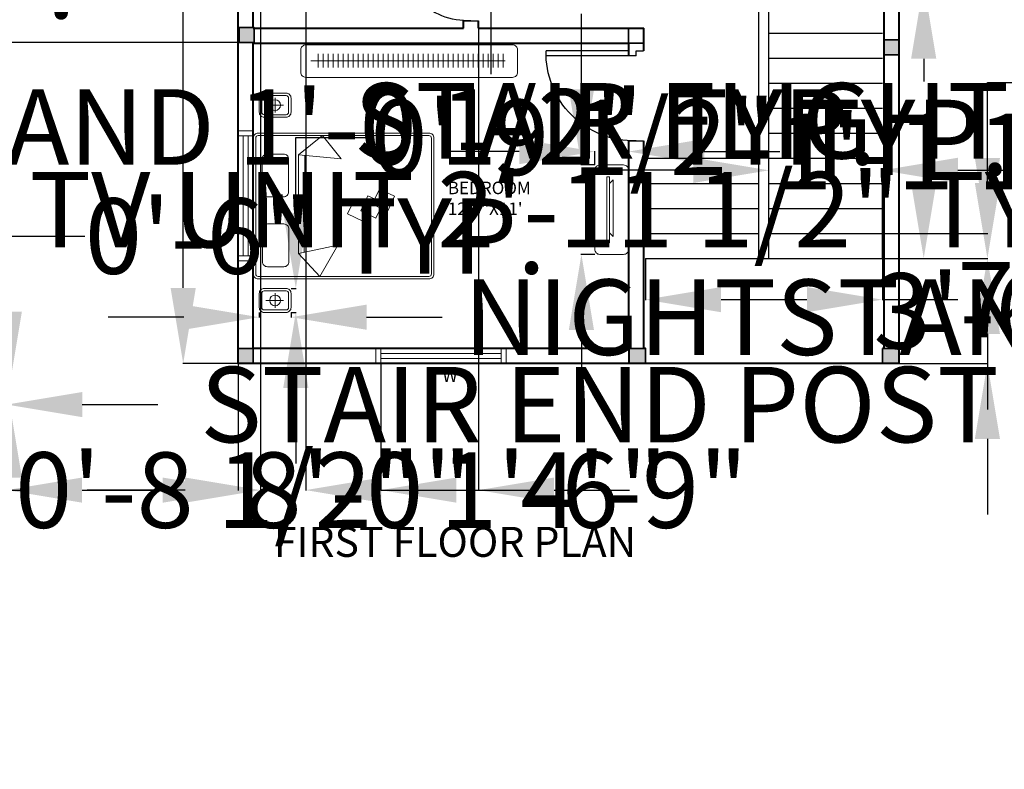
# Model space of a CAD drawing. Units: inches. Extents: x 7323 to 9737, y 2037 to 3322.
# Tile 7 of 19: x 8921 to 9314, y 2037 to 2337. Entities that reach past the tile are written whole.
import ezdxf

# ---------------------------------------------------------------- set-up
doc = ezdxf.new("R2010")
doc.units = ezdxf.units.IN
doc.header["$MEASUREMENT"] = 0
for name, color, linetype, lineweight in [('A-ANNO-DIMS', 2, 'Continuous', 18), ('A-ANNO-TEXT', 7, 'Continuous', 25), ('A-AREA-IDEN', 7, 'Continuous', 18), ('A-COLS', 1, 'Continuous', 35), ('A-DOOR', 4, 'Continuous', 25), ('A-FLOR-CASE', 9, 'Continuous', 20), ('A-FLOR-CASE-PATT', 8, 'Continuous', 13), ('A-FLOR-STRS', 7, 'Continuous', 25), ('A-FURN', 8, 'Continuous', 18), ('A-GLAZ', 4, 'Continuous', 18), ('A-WALL', 7, 'Continuous', 40)]:
    doc.layers.add(name, color=color, linetype=linetype, lineweight=lineweight)
doc.layers.add('A-COLS-PATT', color=18, linetype='Continuous', lineweight=13, true_color=0x000000)
doc.styles.get("Standard").update_dxf_attribs({"font": 'arial.ttf'})
doc.dimstyles.get("Standard").update_dxf_attribs({"dimtxt": 30.18, "dimasz": 30.18, "dimexe": 0.18, "dimexo": 0.0625, "dimgap": 0.09, "dimtad": 0, "dimtih": 1, "dimtoh": 1, "dimdec": 0, "dimzin": 0, "dimdsep": 46, "dimlunit": 3, "dimtxsty": 'Standard', "dimcen": 0.09, "dimadec": 0, "dimazin": 0, "dimtfac": 1, "dimtdec": 0, "dimtofl": 0, "dimtmove": 0, "dimatfit": 3, "dimfxl": 1, "dimtolj": 1, "dimtzin": 0, "dimarcsym": 0})

# ---------------------------------------------------------------- blocks, each defined once
blk = doc.blocks.new('*D11')
at = {"layer": 'A-ANNO-DIMS', "color": 0, "lineweight": -2, "transparency": 16777216}
for p, q in [((9007.88, 2687.3), (8985.8, 2687.3)), ((8985.98, 2657.12), (8985.98, 2458.79)), ((8985.98, 2229.48), (8985.98, 2427.8)), ((9007.88, 2199.3), (8985.8, 2199.3))]:
    blk.add_line(p, q, dxfattribs=at)
at = {"layer": 'A-ANNO-DIMS', "color": 0, "transparency": 16777216}
for points in [[(8980.95, 2657.12), (8991.01, 2657.12), (8985.98, 2687.3)], [(8980.95, 2229.48), (8991.01, 2229.48), (8985.98, 2199.3)]]:
    blk.add_solid(points, dxfattribs=at)
at = {"layer": 'Defpoints', "color": 0, "transparency": 16777216}
for p in [(9007.95, 2687.3), (8985.98, 2199.3), (9007.95, 2199.3)]:
    blk.add_point(p, dxfattribs=at)
at = {"layer": 'A-ANNO-DIMS', "color": 0, "transparency": 16777216, "insert": (8985.98, 2443.3), "char_height": 30.18, "attachment_point": 5}
blk.add_mtext('\\A1;40\'-8"', dxfattribs=at)
blk = doc.blocks.new('WIN-48')
for p, q in [((0, 0), (0, 6)), ((2, 0), (2, 6)), ((2, 4), (50, 4)), ((50, 0), (50, 6)), ((52, 0), (52, 6)), ((2, 2), (50, 2))]:
    blk.add_line(p, q)
blk = doc.blocks.new('STAIR-RETURN-FLIGHT')
for p, q in [((45.32, 110), (94.63, 110)), ((45.32, 0), (45.32, 110)), ((49.32, 0), (49.32, 110)), ((49.32, 100), (94.63, 100)), ((49.32, 90), (94.63, 90)), ((49.32, 80), (94.63, 80)), ((49.32, 70), (94.63, 70)), ((49.32, 60), (94.63, 60)), ((49.32, 50), (94.63, 50)), ((0, 40), (45.32, 40)), ((49.32, 40), (94.63, 40)), ((0, 30), (45.32, 30)), ((49.32, 30), (94.63, 30)), ((0, 20), (45.32, 20)), ((49.32, 20), (94.63, 20)), ((0, 10), (45.32, 10)), ((49.32, 10), (94.63, 10)), ((0, 0), (94.63, 0))]:
    blk.add_line(p, q)
blk = doc.blocks.new('DOOR-36')
for p, q in [((33.01, 39), (39.01, 39)), ((36.01, 5), (0.01, 5)), ((36.01, 5), (36.01, 3)), ((33.01, 3), (0.01, 3)), ((36.01, 3), (39.01, 3)), ((33.01, 0), (39.01, 0))]:
    blk.add_line(p, q)
blk.add_arc((35.01, 4), 35.01, 88.3634, 181.6366)
blk = doc.blocks.new('DOOR-30')
for p, q in [((27.01, 33), (33.01, 33)), ((30.01, 5), (0.01, 5)), ((30.01, 5), (30.01, 3)), ((27.01, 3), (0.01, 3)), ((30.01, 3), (33.01, 3)), ((27.01, 0), (33.01, 0))]:
    blk.add_line(p, q)
blk.add_arc((29.01, 4), 29.02, 88.0251, 181.9749)
blk = doc.blocks.new('MEDIA-CONSOLE')
for p, q in [((5.81, 28.29), (7.29, 29.79)), ((7.29, 29.79), (7.29, 7.16)), ((7.29, 7.16), (5.81, 8.58))]:
    blk.add_line(p, q)
blk.add_lwpolyline([(13.51, 33.75, 0.414214), (11.51, 35.75), (2, 35.75, 0.414214), (0, 33.75), (0, 2, 0.414214), (2, 0), (11.51, 0, 0.414214), (13.51, 2)], format="xyb", close=True)
blk.add_lwpolyline([(5.81, 30.96), (5.81, 30.96), (4.8, 30.96), (4.8, 30.96), (4.8, 4.61), (4.8, 4.61), (5.81, 4.61), (5.81, 4.61)], close=True)
blk = doc.blocks.new('NIGHTSTAND-COMPACT-II')
for p, q in [((2.65, 4.81), (9.72, 4.81)), ((6.35, 7.74), (6.35, 1.85))]:
    blk.add_line(p, q)
for points in [[(0, 7.61, -0.414214), (2, 9.61), (10.71, 9.61, -0.414214), (12.71, 7.61), (12.71, 2, -0.414214), (10.71, 0), (2, 0, -0.414214), (0, 2)], [(1, 7.61, -0.414214), (2, 8.61), (10.71, 8.61, -0.414214), (11.71, 7.61), (11.71, 2, -0.414214), (10.71, 1), (2, 1, -0.414214), (1, 2)]]:
    blk.add_lwpolyline(points, format="xyb", close=True)
blk.add_circle((6.35, 4.81), 2.16)
blk = doc.blocks.new('COL-PLAN-6IN')
blk.add_lwpolyline([(0, 6), (0, 6), (6.06, 6), (6.06, 6), (6.06, 0), (6.06, 0), (0, 0), (0, 0)], close=True)
blk = doc.blocks.new('COL-STAIR-END')
blk.add_lwpolyline([(0, 6), (6.74, 6), (6.74, 0), (0, 0)], close=True)
blk = doc.blocks.new('*D41')
at = {"layer": 'A-ANNO-DIMS', "color": 0, "lineweight": -2, "transparency": 16777216}
for p, q in [((8661.59, 2428.04), (8661.59, 2458.22)), ((8661.59, 2458.22), (8691.77, 2458.22)), ((8657.46, 2397.86), (8661.77, 2397.86)), ((8657.46, 2369.86), (8661.77, 2369.86)), ((8661.59, 2339.68), (8661.59, 2309.5))]:
    blk.add_line(p, q, dxfattribs=at)
at = {"layer": 'A-ANNO-DIMS', "color": 0, "transparency": 16777216}
for points in [[(8656.56, 2428.04), (8666.62, 2428.04), (8661.59, 2397.86)], [(8656.56, 2339.68), (8666.62, 2339.68), (8661.59, 2369.86)]]:
    blk.add_solid(points, dxfattribs=at)
at = {"layer": 'Defpoints', "color": 0, "transparency": 16777216}
for p in [(8657.39, 2397.86), (8661.59, 2397.86), (8657.39, 2369.86)]:
    blk.add_point(p, dxfattribs=at)
at = {"layer": 'A-ANNO-DIMS', "color": 0, "transparency": 16777216, "insert": (8945.06, 2458.22), "char_height": 30.18, "attachment_point": 5}
blk.add_mtext('\\A1;VENT WINDOW 2\'-4" TYP.', dxfattribs=at)
blk = doc.blocks.new('*D43')
at = {"layer": 'A-ANNO-DIMS', "color": 0, "lineweight": -2, "transparency": 16777216}
for p, q in [((9108.94, 2438.75), (9108.94, 2468.93)), ((9104.01, 2408.57), (9109.12, 2408.57)), ((9104.01, 2375.3), (9109.12, 2375.3)), ((9108.94, 2345.12), (9108.94, 2314.94))]:
    blk.add_line(p, q, dxfattribs=at)
at = {"layer": 'A-ANNO-DIMS', "color": 0, "transparency": 16777216}
for points in [[(9103.91, 2438.75), (9113.97, 2438.75), (9108.94, 2408.57)], [(9103.91, 2345.12), (9113.97, 2345.12), (9108.94, 2375.3)]]:
    blk.add_solid(points, dxfattribs=at)
at = {"layer": 'Defpoints', "color": 0, "transparency": 16777216}
for p in [(9103.95, 2408.57), (9108.94, 2408.57), (9103.95, 2375.3)]:
    blk.add_point(p, dxfattribs=at)
at = {"layer": 'A-ANNO-DIMS', "color": 0, "transparency": 16777216, "insert": (9108.94, 2391.93), "char_height": 30.18, "attachment_point": 5}
blk.add_mtext('\\A1;BATH DOOR 2\'-9 1/2" TYP.', dxfattribs=at)
blk = doc.blocks.new('*D44')
at = {"layer": 'A-ANNO-DIMS', "color": 0, "lineweight": -2, "transparency": 16777216}
for p, q in [((9070.67, 2375.23), (9070.67, 2370.12)), ((9103.95, 2375.23), (9103.95, 2370.12)), ((9040.49, 2370.3), (9010.31, 2370.3)), ((9134.13, 2370.3), (9164.31, 2370.3))]:
    blk.add_line(p, q, dxfattribs=at)
at = {"layer": 'A-ANNO-DIMS', "color": 0, "transparency": 16777216}
for points in [[(9040.49, 2375.33), (9040.49, 2365.27), (9070.67, 2370.3)], [(9134.13, 2375.33), (9134.13, 2365.27), (9103.95, 2370.3)]]:
    blk.add_solid(points, dxfattribs=at)
at = {"layer": 'Defpoints', "color": 0, "transparency": 16777216}
for p in [(9070.67, 2375.3), (9103.95, 2375.3), (9103.95, 2370.3)]:
    blk.add_point(p, dxfattribs=at)
at = {"layer": 'A-ANNO-DIMS', "color": 0, "transparency": 16777216, "insert": (9291.8, 2370.3), "char_height": 30.18, "attachment_point": 5}
blk.add_mtext('\\A1;2\'-9 1/2" TYP.', dxfattribs=at)
blk = doc.blocks.new('*D49')
at = {"layer": 'A-ANNO-DIMS', "color": 0, "lineweight": -2, "transparency": 16777216}
for p, q in [((8908.77, 2183.8), (8908.77, 2182.67)), ((8915.5, 2183.8), (8915.5, 2182.67)), ((8878.59, 2182.85), (8848.41, 2182.85)), ((8945.68, 2182.85), (8975.86, 2182.85))]:
    blk.add_line(p, q, dxfattribs=at)
at = {"layer": 'A-ANNO-DIMS', "color": 0, "transparency": 16777216}
for points in [[(8878.59, 2187.88), (8878.59, 2177.82), (8908.77, 2182.85)], [(8945.68, 2187.88), (8945.68, 2177.82), (8915.5, 2182.85)]]:
    blk.add_solid(points, dxfattribs=at)
at = {"layer": 'Defpoints', "color": 0, "transparency": 16777216}
for p in [(8908.77, 2183.86), (8915.5, 2183.86), (8915.5, 2182.85)]:
    blk.add_point(p, dxfattribs=at)
at = {"layer": 'A-ANNO-DIMS', "color": 0, "transparency": 16777216, "insert": (9284.58, 2182.85), "char_height": 30.18, "attachment_point": 5}
blk.add_mtext('\\A1;STAIR END POST 0\'-6 1/2" TYP.', dxfattribs=at)
blk = doc.blocks.new('*D50')
at = {"layer": 'A-ANNO-DIMS', "color": 0, "lineweight": -2, "transparency": 16777216}
for p, q in [((8916.51, 2220.04), (8916.51, 2250.22)), ((8916.51, 2250.22), (8946.69, 2250.22)), ((8915.57, 2189.86), (8916.69, 2189.86)), ((8915.57, 2183.86), (8916.69, 2183.86)), ((8916.51, 2153.68), (8916.51, 2123.5))]:
    blk.add_line(p, q, dxfattribs=at)
at = {"layer": 'A-ANNO-DIMS', "color": 0, "transparency": 16777216}
for points in [[(8911.48, 2220.04), (8921.54, 2220.04), (8916.51, 2189.86)], [(8911.48, 2153.68), (8921.54, 2153.68), (8916.51, 2183.86)]]:
    blk.add_solid(points, dxfattribs=at)
at = {"layer": 'Defpoints', "color": 0, "transparency": 16777216}
for p in [(8915.5, 2189.86), (8916.51, 2189.86), (8915.5, 2183.86)]:
    blk.add_point(p, dxfattribs=at)
at = {"layer": 'A-ANNO-DIMS', "color": 0, "transparency": 16777216, "insert": (9038.77, 2250.22), "char_height": 30.18, "attachment_point": 5}
blk.add_mtext('\\A1;0\'-6" TYP.', dxfattribs=at)
blk = doc.blocks.new('*D55')
at = {"layer": 'A-ANNO-DIMS', "color": 0, "lineweight": -2, "transparency": 16777216}
for p, q in [((9265.38, 2351.3), (9282, 2351.3)), ((9281.82, 2321.12), (9281.82, 2311.99)), ((9281.82, 2271.48), (9281.82, 2280.6)), ((9265.38, 2241.3), (9282, 2241.3))]:
    blk.add_line(p, q, dxfattribs=at)
at = {"layer": 'A-ANNO-DIMS', "color": 0, "transparency": 16777216}
for points in [[(9276.79, 2321.12), (9286.85, 2321.12), (9281.82, 2351.3)], [(9276.79, 2271.48), (9286.85, 2271.48), (9281.82, 2241.3)]]:
    blk.add_solid(points, dxfattribs=at)
at = {"layer": 'Defpoints', "color": 0, "transparency": 16777216}
for p in [(9265.32, 2351.3), (9281.82, 2351.3), (9265.32, 2241.3)]:
    blk.add_point(p, dxfattribs=at)
at = {"layer": 'A-ANNO-DIMS', "color": 0, "transparency": 16777216, "insert": (9281.82, 2296.3), "char_height": 30.18, "attachment_point": 5}
blk.add_mtext('\\A1;STAIR FLIGHT 9\'-2" TYP.', dxfattribs=at)
blk = doc.blocks.new('*D56')
at = {"layer": 'A-ANNO-DIMS', "color": 0, "lineweight": -2, "transparency": 16777216}
for p, q in [((9170.68, 2241.23), (9170.68, 2224.62)), ((9265.32, 2241.23), (9265.32, 2224.62)), ((9200.86, 2224.8), (9235.14, 2224.8)), ((9265.32, 2224.8), (9295.5, 2224.8))]:
    blk.add_line(p, q, dxfattribs=at)
at = {"layer": 'A-ANNO-DIMS', "color": 0, "transparency": 16777216}
for points in [[(9200.86, 2229.83), (9200.86, 2219.77), (9170.68, 2224.8)], [(9235.14, 2229.83), (9235.14, 2219.77), (9265.32, 2224.8)]]:
    blk.add_solid(points, dxfattribs=at)
at = {"layer": 'Defpoints', "color": 0, "transparency": 16777216}
for p in [(9170.68, 2241.3), (9265.32, 2241.3), (9265.32, 2224.8)]:
    blk.add_point(p, dxfattribs=at)
at = {"layer": 'A-ANNO-DIMS', "color": 0, "transparency": 16777216, "insert": (9434.33, 2224.8), "char_height": 30.18, "attachment_point": 5}
blk.add_mtext('\\A1;7\'-10 1/2" TYP.', dxfattribs=at)
blk = doc.blocks.new('*D67')
at = {"layer": 'A-ANNO-DIMS', "color": 0, "lineweight": -2, "transparency": 16777216}
for p, q in [((9145.07, 2308.82), (9145.07, 2339)), ((9150.37, 2278.64), (9144.89, 2278.64)), ((9150.37, 2242.89), (9144.89, 2242.89)), ((9145.07, 2212.71), (9145.07, 2182.53))]:
    blk.add_line(p, q, dxfattribs=at)
at = {"layer": 'A-ANNO-DIMS', "color": 0, "transparency": 16777216}
for points in [[(9140.04, 2308.82), (9150.1, 2308.82), (9145.07, 2278.64)], [(9140.04, 2212.71), (9150.1, 2212.71), (9145.07, 2242.89)]]:
    blk.add_solid(points, dxfattribs=at)
at = {"layer": 'Defpoints', "color": 0, "transparency": 16777216}
for p in [(9145.07, 2278.64), (9150.44, 2278.64), (9150.44, 2242.89)]:
    blk.add_point(p, dxfattribs=at)
at = {"layer": 'A-ANNO-DIMS', "color": 0, "transparency": 16777216, "insert": (9145.07, 2260.76), "char_height": 30.18, "attachment_point": 5}
blk.add_mtext('\\A1;TV UNIT 2\'-11 1/2" TYP.', dxfattribs=at)
blk = doc.blocks.new('*D68')
at = {"layer": 'A-ANNO-DIMS', "color": 0, "lineweight": -2, "transparency": 16777216}
for p, q in [((9120.26, 2284), (9090.08, 2284)), ((9150.44, 2278.7), (9150.44, 2284.18)), ((9163.95, 2278.7), (9163.95, 2284.18)), ((9194.13, 2284), (9224.31, 2284))]:
    blk.add_line(p, q, dxfattribs=at)
at = {"layer": 'A-ANNO-DIMS', "color": 0, "transparency": 16777216}
for points in [[(9120.26, 2289.03), (9120.26, 2278.97), (9150.44, 2284)], [(9194.13, 2289.03), (9194.13, 2278.97), (9163.95, 2284)]]:
    blk.add_solid(points, dxfattribs=at)
at = {"layer": 'Defpoints', "color": 0, "transparency": 16777216}
for p in [(9163.95, 2284), (9150.44, 2278.64), (9163.95, 2278.64)]:
    blk.add_point(p, dxfattribs=at)
at = {"layer": 'A-ANNO-DIMS', "color": 0, "transparency": 16777216, "insert": (9350.12, 2284), "char_height": 30.18, "attachment_point": 5}
blk.add_mtext('\\A1;1\'-1 1/2" TYP.', dxfattribs=at)
blk = doc.blocks.new('*D75')
at = {"layer": 'A-ANNO-DIMS', "color": 0, "lineweight": -2, "transparency": 16777216}
for p, q in [((8629.63, 2293.84), (8599.45, 2293.84)), ((8659.81, 2292), (8659.81, 2294.02)), ((8672.52, 2292), (8672.52, 2294.02)), ((8702.7, 2293.84), (8732.88, 2293.84))]:
    blk.add_line(p, q, dxfattribs=at)
at = {"layer": 'A-ANNO-DIMS', "color": 0, "transparency": 16777216}
for points in [[(8629.63, 2298.87), (8629.63, 2288.81), (8659.81, 2293.84)], [(8702.7, 2298.87), (8702.7, 2288.81), (8672.52, 2293.84)]]:
    blk.add_solid(points, dxfattribs=at)
at = {"layer": 'Defpoints', "color": 0, "transparency": 16777216}
for p in [(8672.52, 2293.84), (8659.81, 2291.93), (8672.52, 2291.93)]:
    blk.add_point(p, dxfattribs=at)
at = {"layer": 'A-ANNO-DIMS', "color": 0, "transparency": 16777216, "insert": (9002.27, 2293.84), "char_height": 30.18, "attachment_point": 5}
blk.add_mtext('\\A1;NIGHTSTAND 1\'-0 1/2" TYP.', dxfattribs=at)
blk = doc.blocks.new('*D76')
at = {"layer": 'A-ANNO-DIMS', "color": 0, "lineweight": -2, "transparency": 16777216}
for p, q in [((8657.91, 2322.11), (8657.91, 2352.29)), ((8657.91, 2352.29), (8688.09, 2352.29)), ((8659.75, 2291.93), (8657.73, 2291.93)), ((8659.75, 2282.32), (8657.73, 2282.32)), ((8657.91, 2252.14), (8657.91, 2221.96))]:
    blk.add_line(p, q, dxfattribs=at)
at = {"layer": 'A-ANNO-DIMS', "color": 0, "transparency": 16777216}
for points in [[(8652.88, 2322.11), (8662.94, 2322.11), (8657.91, 2291.93)], [(8652.88, 2252.14), (8662.94, 2252.14), (8657.91, 2282.32)]]:
    blk.add_solid(points, dxfattribs=at)
at = {"layer": 'Defpoints', "color": 0, "transparency": 16777216}
for p in [(8657.91, 2291.93), (8659.81, 2291.93), (8659.81, 2282.32)]:
    blk.add_point(p, dxfattribs=at)
at = {"layer": 'A-ANNO-DIMS', "color": 0, "transparency": 16777216, "insert": (8815.32, 2352.29), "char_height": 30.18, "attachment_point": 5}
blk.add_mtext('\\A1;0\'-9 1/2" TYP.', dxfattribs=at)
blk = doc.blocks.new('*D77')
at = {"layer": 'A-ANNO-DIMS', "color": 0, "lineweight": -2, "transparency": 16777216}
for p, q in [((9016.36, 2219.63), (9016.36, 2217.61)), ((9029.07, 2219.63), (9029.07, 2217.61)), ((8986.18, 2217.79), (8956, 2217.79)), ((9059.25, 2217.79), (9089.43, 2217.79))]:
    blk.add_line(p, q, dxfattribs=at)
at = {"layer": 'A-ANNO-DIMS', "color": 0, "transparency": 16777216}
for points in [[(8986.18, 2222.82), (8986.18, 2212.76), (9016.36, 2217.79)], [(9059.25, 2222.82), (9059.25, 2212.76), (9029.07, 2217.79)]]:
    blk.add_solid(points, dxfattribs=at)
at = {"layer": 'Defpoints', "color": 0, "transparency": 16777216}
for p in [(9016.36, 2219.69), (9029.07, 2219.69), (9029.07, 2217.79)]:
    blk.add_point(p, dxfattribs=at)
at = {"layer": 'A-ANNO-DIMS', "color": 0, "transparency": 16777216, "insert": (9358.82, 2217.79), "char_height": 30.18, "attachment_point": 5}
blk.add_mtext('\\A1;NIGHTSTAND 1\'-0 1/2" TYP.', dxfattribs=at)
blk = doc.blocks.new('*D78')
at = {"layer": 'A-ANNO-DIMS', "color": 0, "lineweight": -2, "transparency": 16777216}
for p, q in [((9030.98, 2259.48), (9030.98, 2289.66)), ((9030.98, 2289.66), (9061.16, 2289.66)), ((9029.14, 2229.3), (9031.16, 2229.3)), ((9029.14, 2219.69), (9031.16, 2219.69)), ((9030.98, 2189.51), (9030.98, 2159.33))]:
    blk.add_line(p, q, dxfattribs=at)
at = {"layer": 'A-ANNO-DIMS', "color": 0, "transparency": 16777216}
for points in [[(9025.95, 2259.48), (9036.01, 2259.48), (9030.98, 2229.3)], [(9025.95, 2189.51), (9036.01, 2189.51), (9030.98, 2219.69)]]:
    blk.add_solid(points, dxfattribs=at)
at = {"layer": 'Defpoints', "color": 0, "transparency": 16777216}
for p in [(9029.07, 2229.3), (9030.98, 2229.3), (9029.07, 2219.69)]:
    blk.add_point(p, dxfattribs=at)
at = {"layer": 'A-ANNO-DIMS', "color": 0, "transparency": 16777216, "insert": (9188.39, 2289.66), "char_height": 30.18, "attachment_point": 5}
blk.add_mtext('\\A1;0\'-9 1/2" TYP.', dxfattribs=at)
blk = doc.blocks.new('*D79')
at = {"layer": 'A-ANNO-DIMS', "color": 0, "lineweight": -2, "transparency": 16777216}
for p, q in [((8871.1, 2395.97), (8871.1, 2394.46)), ((8880.36, 2395.97), (8880.36, 2394.46)), ((8840.92, 2394.64), (8810.74, 2394.64)), ((8910.54, 2394.64), (8940.72, 2394.64))]:
    blk.add_line(p, q, dxfattribs=at)
at = {"layer": 'A-ANNO-DIMS', "color": 0, "transparency": 16777216}
for points in [[(8840.92, 2399.67), (8840.92, 2389.61), (8871.1, 2394.64)], [(8910.54, 2399.67), (8910.54, 2389.61), (8880.36, 2394.64)]]:
    blk.add_solid(points, dxfattribs=at)
at = {"layer": 'Defpoints', "color": 0, "transparency": 16777216}
for p in [(8871.1, 2396.03), (8880.36, 2396.03), (8880.36, 2394.64)]:
    blk.add_point(p, dxfattribs=at)
at = {"layer": 'A-ANNO-DIMS', "color": 0, "transparency": 16777216, "insert": (9195.57, 2394.64), "char_height": 30.18, "attachment_point": 5}
blk.add_mtext('\\A1;SIDE TABLE 0\'-9 1/2" TYP.', dxfattribs=at)
blk = doc.blocks.new('*D80')
at = {"layer": 'A-ANNO-DIMS', "color": 0, "lineweight": -2, "transparency": 16777216}
for p, q in [((8881.74, 2435.12), (8881.74, 2465.3)), ((8881.74, 2465.3), (8911.92, 2465.3)), ((8880.42, 2404.94), (8881.92, 2404.94)), ((8880.42, 2396.03), (8881.92, 2396.03)), ((8881.74, 2365.85), (8881.74, 2335.67))]:
    blk.add_line(p, q, dxfattribs=at)
at = {"layer": 'A-ANNO-DIMS', "color": 0, "transparency": 16777216}
for points in [[(8876.71, 2435.12), (8886.77, 2435.12), (8881.74, 2404.94)], [(8876.71, 2365.85), (8886.77, 2365.85), (8881.74, 2396.03)]]:
    blk.add_solid(points, dxfattribs=at)
at = {"layer": 'Defpoints', "color": 0, "transparency": 16777216}
for p in [(8880.36, 2404.94), (8881.74, 2404.94), (8880.36, 2396.03)]:
    blk.add_point(p, dxfattribs=at)
at = {"layer": 'A-ANNO-DIMS', "color": 0, "transparency": 16777216, "insert": (9003.99, 2465.3), "char_height": 30.18, "attachment_point": 5}
blk.add_mtext('\\A1;0\'-9" TYP.', dxfattribs=at)
blk = doc.blocks.new('*D97')
at = {"layer": 'A-ANNO-DIMS', "color": 0, "lineweight": -2, "transparency": 16777216}
for p, q in [((8813.39277, 2308.800309), (8813.39277, 2148.482809)), ((8915.39277, 2183.800309), (8915.39277, 2148.482809)), ((8783.21277, 2148.662809), (8753.03277, 2148.662809)), ((8945.57277, 2148.662809), (8975.75277, 2148.662809))]:
    blk.add_line(p, q, dxfattribs=at)
at = {"layer": 'A-ANNO-DIMS', "color": 0, "transparency": 16777216}
for points in [[(8783.21277, 2153.692809), (8783.21277, 2143.632809), (8813.39277, 2148.662809)], [(8945.57277, 2153.692809), (8945.57277, 2143.632809), (8915.39277, 2148.662809)]]:
    blk.add_solid(points, dxfattribs=at)
at = {"layer": 'Defpoints', "color": 0, "transparency": 16777216}
for p in [(8813.39277, 2308.862809), (8915.39277, 2183.862809), (8915.39277, 2148.662809)]:
    blk.add_point(p, dxfattribs=at)
at = {"layer": 'A-ANNO-DIMS', "color": 0, "transparency": 16777216, "insert": (8864.39277, 2148.662809), "char_height": 30.18, "attachment_point": 5}
blk.add_mtext('\\A1;8\'-6"', dxfattribs=at)
blk = doc.blocks.new('*D99')
at = {"layer": 'A-ANNO-DIMS', "color": 0, "lineweight": -2, "transparency": 16777216}
for p, q in [((9007.95, 2199.23), (9007.95, 2148.48)), ((9064.95, 2199.23), (9064.95, 2148.48)), ((8977.77, 2148.66), (8947.59, 2148.66)), ((9095.13, 2148.66), (9125.31, 2148.66))]:
    blk.add_line(p, q, dxfattribs=at)
at = {"layer": 'A-ANNO-DIMS', "color": 0, "transparency": 16777216}
for points in [[(8977.77, 2153.69), (8977.77, 2143.63), (9007.95, 2148.66)], [(9095.13, 2153.69), (9095.13, 2143.63), (9064.95, 2148.66)]]:
    blk.add_solid(points, dxfattribs=at)
at = {"layer": 'Defpoints', "color": 0, "transparency": 16777216}
for p in [(9007.95, 2199.3), (9064.95, 2199.3), (9064.95, 2148.66)]:
    blk.add_point(p, dxfattribs=at)
at = {"layer": 'A-ANNO-DIMS', "color": 0, "transparency": 16777216, "insert": (9166.12, 2148.66), "char_height": 30.18, "attachment_point": 5}
blk.add_mtext('\\A1;4\'-9"', dxfattribs=at)
blk = doc.blocks.new('*D105')
at = {"layer": 'A-ANNO-DIMS', "color": 0, "lineweight": -2, "transparency": 16777216}
for p, q in [((9007.945402, 2365.232705), (9007.945402, 2148.482809)), ((9103.945402, 2333.232705), (9103.945402, 2148.482809)), ((8977.765402, 2148.662809), (8947.585402, 2148.662809)), ((9134.125402, 2148.662809), (9164.305402, 2148.662809))]:
    blk.add_line(p, q, dxfattribs=at)
at = {"layer": 'A-ANNO-DIMS', "color": 0, "transparency": 16777216}
for points in [[(8977.765402, 2153.692809), (8977.765402, 2143.632809), (9007.945402, 2148.662809)], [(9134.125402, 2153.692809), (9134.125402, 2143.632809), (9103.945402, 2148.662809)]]:
    blk.add_solid(points, dxfattribs=at)
at = {"layer": 'Defpoints', "color": 0, "transparency": 16777216}
for p in [(9007.945402, 2365.295205), (9103.945402, 2333.295205), (9103.945402, 2148.662809)]:
    blk.add_point(p, dxfattribs=at)
at = {"layer": 'A-ANNO-DIMS', "color": 0, "transparency": 16777216, "insert": (9055.945402, 2148.662809), "char_height": 30.18, "attachment_point": 5}
blk.add_mtext('\\A1;8\'-0"', dxfattribs=at)
blk = doc.blocks.new('*D106')
at = {"layer": 'A-ANNO-DIMS', "color": 0, "lineweight": -2, "transparency": 16777216}
for p, q in [((9008.12, 2519.31), (8587.16, 2519.31)), ((8587.34, 2489.13), (8587.34, 2439.14)), ((8587.34, 2357.76), (8587.34, 2407.75)), ((9008.23, 2327.58), (8587.16, 2327.58))]:
    blk.add_line(p, q, dxfattribs=at)
at = {"layer": 'A-ANNO-DIMS', "color": 0, "transparency": 16777216}
for points in [[(8582.31, 2489.13), (8592.37, 2489.13), (8587.34, 2519.31)], [(8582.31, 2357.76), (8592.37, 2357.76), (8587.34, 2327.58)]]:
    blk.add_solid(points, dxfattribs=at)
at = {"layer": 'Defpoints', "color": 0, "transparency": 16777216}
for p in [(8587.34, 2519.31), (9008.18, 2519.31), (9008.29, 2327.58)]:
    blk.add_point(p, dxfattribs=at)
at = {"layer": 'A-ANNO-DIMS', "color": 0, "transparency": 16777216, "insert": (8587.34, 2423.44), "char_height": 30.18, "attachment_point": 5}
blk.add_mtext('\\A1;15\'-11 1/2"', dxfattribs=at)
blk = doc.blocks.new('*D107')
at = {"layer": 'A-ANNO-DIMS', "color": 0, "lineweight": -2, "transparency": 16777216}
for p, q in [((8855.74, 2420.27), (8855.74, 2148.48)), ((8864.06, 2412.89), (8864.06, 2148.48)), ((8825.56, 2148.66), (8795.38, 2148.66)), ((8894.24, 2148.66), (8924.42, 2148.66))]:
    blk.add_line(p, q, dxfattribs=at)
at = {"layer": 'A-ANNO-DIMS', "color": 0, "transparency": 16777216}
for points in [[(8825.56, 2153.69), (8825.56, 2143.63), (8855.74, 2148.66)], [(8894.24, 2153.69), (8894.24, 2143.63), (8864.06, 2148.66)]]:
    blk.add_solid(points, dxfattribs=at)
at = {"layer": 'Defpoints', "color": 0, "transparency": 16777216}
for p in [(8855.74, 2420.33), (8864.06, 2412.95), (8864.06, 2148.66)]:
    blk.add_point(p, dxfattribs=at)
at = {"layer": 'A-ANNO-DIMS', "color": 0, "transparency": 16777216, "insert": (8999.78, 2148.66), "char_height": 30.18, "attachment_point": 5}
blk.add_mtext('\\A1;0\'-8 1/2"', dxfattribs=at)
blk = doc.blocks.new('*D109')
at = {"layer": 'A-ANNO-DIMS', "color": 0, "lineweight": -2, "transparency": 16777216}
for p, q in [((9016.91, 2377.23), (9016.91, 2148.48)), ((9034.93, 2377.23), (9034.93, 2148.48)), ((8986.73, 2148.66), (8956.55, 2148.66)), ((9065.11, 2148.66), (9095.29, 2148.66))]:
    blk.add_line(p, q, dxfattribs=at)
at = {"layer": 'A-ANNO-DIMS', "color": 0, "transparency": 16777216}
for points in [[(8986.73, 2153.69), (8986.73, 2143.63), (9016.91, 2148.66)], [(9065.11, 2153.69), (9065.11, 2143.63), (9034.93, 2148.66)]]:
    blk.add_solid(points, dxfattribs=at)
at = {"layer": 'Defpoints', "color": 0, "transparency": 16777216}
for p in [(9016.91, 2377.3), (9034.93, 2377.3), (9034.93, 2148.66)]:
    blk.add_point(p, dxfattribs=at)
at = {"layer": 'A-ANNO-DIMS', "color": 0, "transparency": 16777216, "insert": (9134.07, 2148.66), "char_height": 30.18, "attachment_point": 5}
blk.add_mtext('\\A1;1\'-6"', dxfattribs=at)
blk = doc.blocks.new('*D110')
at = {"layer": 'A-ANNO-DIMS', "color": 0, "lineweight": -2, "transparency": 16777216}
for p, q in [((8587.34, 2449.91), (8587.34, 2480.09)), ((9018.85, 2419.73), (8587.16, 2419.73)), ((9018.85, 2375.3), (8587.16, 2375.3)), ((8587.34, 2345.12), (8587.34, 2314.94))]:
    blk.add_line(p, q, dxfattribs=at)
at = {"layer": 'A-ANNO-DIMS', "color": 0, "transparency": 16777216}
for points in [[(8582.31, 2449.91), (8592.37, 2449.91), (8587.34, 2419.73)], [(8582.31, 2345.12), (8592.37, 2345.12), (8587.34, 2375.3)]]:
    blk.add_solid(points, dxfattribs=at)
at = {"layer": 'Defpoints', "color": 0, "transparency": 16777216}
for p in [(8587.34, 2419.73), (9018.91, 2419.73), (9018.91, 2375.3)]:
    blk.add_point(p, dxfattribs=at)
at = {"layer": 'A-ANNO-DIMS', "color": 0, "transparency": 16777216, "insert": (8587.34, 2397.51), "char_height": 30.18, "attachment_point": 5}
blk.add_mtext('\\A1;3\'-8 1/2"', dxfattribs=at)
blk = doc.blocks.new('*D115')
at = {"layer": 'A-ANNO-DIMS', "color": 0, "lineweight": -2, "transparency": 16777216}
for p, q in [((9307.269962, 2271.475205), (9307.269962, 2301.655205)), ((9265.38043, 2241.295205), (9307.449962, 2241.295205)), ((9265.38043, 2199.295205), (9307.449962, 2199.295205)), ((9307.269962, 2169.115205), (9307.269962, 2138.935205))]:
    blk.add_line(p, q, dxfattribs=at)
at = {"layer": 'A-ANNO-DIMS', "color": 0, "transparency": 16777216}
for points in [[(9302.239962, 2271.475205), (9312.299962, 2271.475205), (9307.269962, 2241.295205)], [(9302.239962, 2169.115205), (9312.299962, 2169.115205), (9307.269962, 2199.295205)]]:
    blk.add_solid(points, dxfattribs=at)
at = {"layer": 'Defpoints', "color": 0, "transparency": 16777216}
for p in [(9265.31793, 2241.295205), (9307.269962, 2241.295205), (9265.31793, 2199.295205)]:
    blk.add_point(p, dxfattribs=at)
at = {"layer": 'A-ANNO-DIMS', "color": 0, "transparency": 16777216, "insert": (9307.269962, 2220.295205), "char_height": 30.18, "attachment_point": 5}
blk.add_mtext('\\A1;3\'-6"', dxfattribs=at)
blk = doc.blocks.new('*D116')
at = {"layer": 'A-ANNO-DIMS', "color": 0, "lineweight": -2, "transparency": 16777216}
for p, q in [((9307.27, 2281.48), (9307.27, 2311.66)), ((9307.27, 2311.66), (9337.45, 2311.66)), ((9265.38, 2251.3), (9307.45, 2251.3)), ((9265.38, 2241.3), (9307.45, 2241.3)), ((9307.27, 2211.12), (9307.27, 2180.94))]:
    blk.add_line(p, q, dxfattribs=at)
at = {"layer": 'A-ANNO-DIMS', "color": 0, "transparency": 16777216}
for points in [[(9302.24, 2281.48), (9312.3, 2281.48), (9307.27, 2251.3)], [(9302.24, 2211.12), (9312.3, 2211.12), (9307.27, 2241.3)]]:
    blk.add_solid(points, dxfattribs=at)
at = {"layer": 'Defpoints', "color": 0, "transparency": 16777216}
for p in [(9265.32, 2251.3), (9307.27, 2251.3), (9265.32, 2241.3)]:
    blk.add_point(p, dxfattribs=at)
at = {"layer": 'A-ANNO-DIMS', "color": 0, "transparency": 16777216, "insert": (9389.38, 2311.66), "char_height": 30.18, "attachment_point": 5}
blk.add_mtext('\\A1;0\'-10"', dxfattribs=at)
blk = doc.blocks.new('*D122')
at = {"layer": 'A-ANNO-DIMS', "color": 0, "lineweight": -2, "transparency": 16777216}
for p, q in [((9189.82, 2276.5), (9159.64, 2276.5)), ((9220, 2241.36), (9220, 2276.68)), ((9265.32, 2241.36), (9265.32, 2276.68)), ((9295.5, 2276.5), (9325.68, 2276.5))]:
    blk.add_line(p, q, dxfattribs=at)
at = {"layer": 'A-ANNO-DIMS', "color": 0, "transparency": 16777216}
for points in [[(9189.82, 2281.53), (9189.82, 2271.47), (9220, 2276.5)], [(9295.5, 2281.53), (9295.5, 2271.47), (9265.32, 2276.5)]]:
    blk.add_solid(points, dxfattribs=at)
at = {"layer": 'Defpoints', "color": 0, "transparency": 16777216}
for p in [(9265.32, 2276.5), (9220, 2241.3), (9265.32, 2241.3)]:
    blk.add_point(p, dxfattribs=at)
at = {"layer": 'A-ANNO-DIMS', "color": 0, "transparency": 16777216, "insert": (9401.03, 2276.5), "char_height": 30.18, "attachment_point": 5}
blk.add_mtext('\\A1;3\'-9 1/2"', dxfattribs=at)

msp = doc.modelspace()

# ---------------------------------------------------------------- hatches: boundary and pattern name
at = {"layer": 'A-COLS-PATT'}
h = msp.add_hatch(color=256, dxfattribs=at)
h.dxf.hatch_style = 1
h.paths.add_polyline_path([(8915.39, 2189.86), (8908.77, 2189.86), (8908.77, 2183.86), (8915.39, 2183.86)])
h.paths.add_polyline_path([(8657.61, 2189.86), (8651.55, 2189.86), (8651.55, 2183.86), (8657.61, 2183.86)])
h.paths.add_polyline_path([(8814.13, 2189.86), (8807.39, 2189.86), (8807.39, 2183.86), (8814.13, 2183.86)])
h.paths.add_polyline_path([(8813.39, 2317.86), (8807.36, 2317.86), (8807.36, 2311.86), (8813.39, 2311.86)])
h.paths.add_polyline_path([(8915.34, 2313.13), (8909.39, 2313.13), (8909.39, 2307.13), (8915.34, 2307.13)])
h.paths.add_polyline_path([(8657.62, 2317.86), (8657.39, 2317.86), (8657.39, 2318.08), (8651.55, 2318.08), (8651.55, 2312.08), (8657.62, 2312.08)])
h.paths.add_polyline_path([(8915.39, 2671.84), (8909.37, 2671.84), (8909.37, 2665.86), (8909.39, 2665.86), (8915.39, 2665.84)])
h.paths.add_polyline_path([(8657.59, 2671.81), (8651.52, 2671.81), (8651.52, 2665.81), (8657.39, 2665.81), (8657.39, 2665.86)])
h.paths.add_polyline_path([(8915.28, 2503.94), (8909.39, 2503.94), (8909.39, 2503.86), (8909.22, 2497.94), (8915.28, 2497.94)])
h.paths.add_polyline_path([(8657.53, 2503.86), (8657.39, 2503.86), (8651.46, 2503.96), (8651.46, 2497.96), (8657.53, 2497.96)])
h.paths.add_polyline_path([(9014.24, 2519.3), (9013.95, 2519.3), (9008.18, 2519.31), (9008.18, 2513.31), (9014.24, 2513.31)])
h.paths.add_polyline_path([(9013.95, 2687.3), (9007.95, 2687.3), (9007.95, 2681.3), (9013.95, 2681.3)])
h.paths.add_polyline_path([(9271.95, 2687.3), (9266.01, 2687.3), (9266.01, 2681.35), (9271.95, 2681.35)])
h.paths.add_polyline_path([(9271.95, 2205.3), (9265.32, 2205.3), (9265.32, 2199.3), (9271.95, 2199.3)])
h.paths.add_polyline_path([(9170.68, 2205.3), (9163.95, 2205.3), (9163.95, 2199.3), (9170.68, 2199.3)])
h.paths.add_polyline_path([(9013.95, 2205.3), (9007.95, 2205.3), (9007.95, 2199.3), (9013.95, 2199.3)])
h.paths.add_polyline_path([(9271.95, 2519.51), (9265.95, 2519.51), (9265.95, 2519.3), (9265.93, 2513.51), (9271.95, 2513.51)])
h.paths.add_polyline_path([(9271.95, 2328.64), (9265.95, 2328.64), (9265.95, 2322.64), (9271.95, 2322.64)])
h.paths.add_polyline_path([(9014.35, 2333.3), (9013.95, 2333.3), (9013.95, 2333.58), (9008.29, 2333.58), (9008.29, 2327.58), (9014.35, 2327.58)])
at = {"layer": 'A-FLOR-CASE-PATT'}
h = msp.add_hatch(dxfattribs=at)
h.set_pattern_fill('ANSI31', color=256, scale=15.99978, angle=45, style=0)
h.paths.add_polyline_path([(9039.85, 2317.56), (9113.91, 2317.56), (9113.91, 2323.12), (9039.85, 2323.12)])

# ---------------------------------------------------------------- linework, layer by layer
at = {"layer": 'A-FLOR-CASE'}
msp.add_line((9036.94, 2320.22), (9114.66, 2320.22), dxfattribs=at)
msp.add_lwpolyline([(9032.96, 2315.67, 0.414214), (9034.96, 2313.67), (9117.59, 2313.67, 0.414214), (9119.59, 2315.67), (9119.59, 2324.65, 0.414214), (9117.59, 2326.65), (9034.96, 2326.65, 0.414214), (9032.96, 2324.65)], format="xyb", close=True, dxfattribs=at)
at = {"layer": 'A-FURN'}
for p, q in [((9031.98, 2282.73), (9041.69, 2290.41)), ((9041.69, 2290.41), (9049.04, 2281.13)), ((9031.98, 2282.73), (9031.98, 2243.21)), ((9049.04, 2281.13), (9031.98, 2282.73)), ((9034.61, 2282.48), (9034.25, 2243.69)), ((9047.72, 2246.53), (9031.98, 2243.21)), ((9040.53, 2234.07), (9047.72, 2246.53)), ((9031.98, 2243.21), (9040.53, 2234.07))]:
    msp.add_line(p, q, dxfattribs=at)
for points in [[(9013.95, 2235.07, 0.414214), (9015.95, 2233.07), (9084.14, 2233.07, 0.414214), (9086.14, 2235.07), (9086.14, 2289.41, 0.414214), (9084.14, 2291.41), (9015.95, 2291.41, 0.414214), (9013.95, 2289.41)], [(9014.95, 2235.07, 0.414214), (9015.95, 2234.07), (9084.14, 2234.07, 0.414214), (9085.14, 2235.07), (9085.14, 2289.41, 0.414214), (9084.14, 2290.41), (9015.95, 2290.41, 0.414214), (9014.95, 2289.41)], [(9017.53, 2281, -0.414214), (9019.53, 2283), (9026.08, 2283, -0.414214), (9028.08, 2281), (9028.08, 2267.91, -0.414214), (9026.08, 2265.91), (9019.53, 2265.91, -0.414214), (9017.53, 2267.91)], [(9017.64, 2253.05, -0.414214), (9019.64, 2255.05), (9026.2, 2255.05, -0.414214), (9028.2, 2253.05), (9028.2, 2239.97, -0.414214), (9026.2, 2237.97), (9019.64, 2237.97, -0.414214), (9017.64, 2239.97)]]:
    msp.add_lwpolyline(points, format="xyb", close=True, dxfattribs=at)
for points in [[(9059.78, 2266.33), (9056.94, 2260.27), (9062.99, 2257.43), (9065.84, 2263.48)], [(9064.36, 2268.97), (9061.52, 2262.92), (9067.57, 2260.07), (9070.42, 2266.13)], [(9054.52, 2265.11), (9051.67, 2259.05), (9057.72, 2256.21), (9060.57, 2262.26)]]:
    msp.add_lwpolyline(points, close=True, dxfattribs=at)
at = {"layer": 'A-WALL'}
for p, q in [((9007.95, 2199.3), (9007.95, 2687.3)), ((9271.95, 2687.3), (9271.95, 2199.3)), ((9265.95, 2513.3), (9265.95, 2205.3)), ((9013.95, 2333.3), (9013.95, 2369.3)), ((9013.95, 2333.3), (9097.95, 2333.3)), ((9097.95, 2333.3), (9097.95, 2336.35)), ((9103.95, 2333.3), (9103.95, 2336.3)), ((9103.95, 2333.3), (9169.95, 2333.3)), ((9169.95, 2324.3), (9169.95, 2333.3)), ((9013.95, 2205.3), (9013.95, 2327.3)), ((9013.95, 2327.3), (9163.95, 2327.3)), ((9163.95, 2322.3), (9163.95, 2327.3)), ((9163.95, 2205.3), (9163.95, 2288.34)), ((9169.95, 2205.3), (9169.95, 2288.3)), ((9163.95, 2205.3), (9013.95, 2205.3)), ((9163.95, 2205.3), (9158.95, 2205.3)), ((9163.95, 2205.3), (9163.95, 2199.3)), ((9170.68, 2205.3), (9169.95, 2205.3)), ((9265.95, 2205.3), (9265.32, 2205.3)), ((9160.95, 2199.3), (9007.95, 2199.3)), ((9271.95, 2199.3), (9160.95, 2199.3))]:
    msp.add_line(p, q, dxfattribs=at)

# ---------------------------------------------------------------- block references
at = {"layer": 'A-COLS'}
for name, p in [('COL-PLAN-6IN', (9008.29, 2327.58)), ('COL-PLAN-6IN', (9163.91, 2327.29)), ('COL-PLAN-6IN', (9265.88, 2322.64)), ('COL-PLAN-6IN', (9007.88, 2199.3)), ('COL-STAIR-END', (9163.95, 2199.3)), ('COL-STAIR-END', (9265.32, 2199.3))]:
    msp.add_blockref(name, p, dxfattribs=at)
at = {"layer": 'A-DOOR', "extrusion": (0, 0, -1), "zscale": -1, "rotation": 180}
for name, p in [('DOOR-30', (-9070.93, 2369.3)), ('DOOR-36', (-9130.93, 2327.29))]:
    msp.add_blockref(name, p, dxfattribs=at)
at = {"layer": 'A-FLOR-STRS'}
msp.add_blockref('STAIR-RETURN-FLIGHT', (9170.68, 2241.3), dxfattribs=at)
at = {"layer": 'A-FURN'}
for name, p in [('NIGHTSTAND-COMPACT-II', (9016.36, 2297.75)), ('MEDIA-CONSOLE', (9150.44, 2242.89)), ('NIGHTSTAND-COMPACT-II', (9016.36, 2219.69))]:
    msp.add_blockref(name, p, dxfattribs=at)
at = {"layer": 'A-GLAZ', "rotation": 270.0000000000041}
msp.add_blockref('WIN-48', (9007.95, 2292.29), dxfattribs=at)
at = {"layer": 'A-GLAZ'}
msp.add_blockref('WIN-48', (9062.95, 2199.3), dxfattribs=at)

# ---------------------------------------------------------------- texts
at = {"layer": 'A-ANNO-TEXT', "attachment_point": 1}
for s, width, insert, char_height in [('W', 26.304, (9089.59, 2196.86), 5), ('FIRST FLOOR PLAN', 222.6475, (9022.19, 2133.98), 12)]:
    msp.add_mtext_dynamic_manual_height_columns(s, width=width, gutter_width=1, heights=[0], dxfattribs=dict(at, insert=insert, char_height=char_height))
at = {"layer": 'A-AREA-IDEN', "insert": (9091.69, 2271.97), "char_height": 5, "attachment_point": 1}
msp.add_mtext_dynamic_manual_height_columns('BEDROOM\\P12\'6"X11\'', width=44.1759, gutter_width=1, heights=[0], dxfattribs=at)

# ---------------------------------------------------------------- dimensions: what is measured, and where the dimension line sits
at = {"layer": 'A-ANNO-DIMS'}
for base, p1, p2, override, picture, middle in [((8985.98, 2199.3), (9007.95, 2687.3), (9007.95, 2199.3), {"dimclrd": 0, "dimclre": 0, "dimclrt": 0}, '*D11', (8985.98, 2443.3)), ((8587.34, 2519.31), (9008.29, 2327.58), (9008.18, 2519.31), {"dimdec": 1, "dimlfac": 1, "dimrnd": 0, "dimzin": 1, "dimdsep": 46, "dimlunit": 4, "dimfrac": 2}, '*D106', (8587.34, 2423.44)), ((8587.34, 2419.73), (9018.91, 2375.3), (9018.91, 2419.73), {"dimdec": 1, "dimlfac": 1, "dimrnd": 0, "dimzin": 1, "dimdsep": 46, "dimlunit": 4, "dimfrac": 2}, '*D110', (8587.34, 2397.51)), ((9307.27, 2251.3), (9265.32, 2241.3), (9265.32, 2251.3), {"dimdec": 1, "dimlfac": 1, "dimrnd": 0, "dimzin": 1, "dimdsep": 46, "dimlunit": 4, "dimfrac": 2}, '*D116', (9389.38, 2311.66)), ((9307.27, 2241.3), (9265.32, 2199.3), (9265.32, 2241.3), {"dimdec": 1, "dimlfac": 1, "dimrnd": 0, "dimzin": 1, "dimdsep": 46, "dimlunit": 4, "dimfrac": 2}, '*D115', (9307.27, 2220.3))]:
    dim = msp.add_linear_dim(base=base, p1=p1, p2=p2, angle=90, dimstyle='Standard', override=override, dxfattribs=at)
    dim.commit()
    dim.dimension.update_dxf_attribs({"geometry": picture, "text_midpoint": middle})
for base, p1, p2, text, picture, middle in [((8661.59, 2397.86), (8657.39, 2369.86), (8657.39, 2397.86), 'VENT WINDOW <> TYP.', '*D41', (8945.06, 2458.22)), ((9108.94, 2408.57), (9103.95, 2375.3), (9103.95, 2408.57), 'BATH DOOR <> TYP.', '*D43', (9108.94, 2391.93)), ((8881.74, 2404.94), (8880.36, 2396.03), (8880.36, 2404.94), '<> TYP.', '*D80', (9003.99, 2465.3)), ((8657.91, 2291.93), (8659.81, 2282.32), (8659.81, 2291.93), '<> TYP.', '*D76', (8815.32, 2352.29)), ((9281.82, 2351.3), (9265.32, 2241.3), (9265.32, 2351.3), 'STAIR FLIGHT <> TYP.', '*D55', (9281.82, 2296.3)), ((9145.0746, 2278.635), (9150.4365, 2242.8889), (9150.4365, 2278.635), 'TV UNIT <> TYP.', '*D67', (9145.0746, 2260.762)), ((9030.98, 2229.3), (9029.07, 2219.69), (9029.07, 2229.3), '<> TYP.', '*D78', (9188.39, 2289.66)), ((8916.51, 2189.86), (8915.5, 2183.86), (8915.5, 2189.86), '<> TYP.', '*D50', (9038.77, 2250.22))]:
    dim = msp.add_linear_dim(base=base, p1=p1, p2=p2, angle=90, text=text, dimstyle='Standard', override={"dimdec": 1, "dimlfac": 1, "dimrnd": 0, "dimzin": 1, "dimdsep": 46, "dimlunit": 4, "dimfrac": 2}, dxfattribs=at)
    dim.commit()
    dim.dimension.update_dxf_attribs({"geometry": picture, "text_midpoint": middle})
for base, p1, p2, text, picture, middle in [((8880.36, 2394.64), (8871.1, 2396.03), (8880.36, 2396.03), 'SIDE TABLE <> TYP.', '*D79', (9195.57, 2394.64)), ((9103.95, 2370.3), (9070.67, 2375.3), (9103.95, 2375.3), '<> TYP.', '*D44', (9291.8, 2370.3)), ((8672.52, 2293.84), (8659.81, 2291.93), (8672.52, 2291.93), 'NIGHTSTAND <> TYP.', '*D75', (9002.27, 2293.84)), ((9163.95, 2284), (9150.44, 2278.64), (9163.95, 2278.64), '<> TYP.', '*D68', (9350.12, 2284)), ((8915.5, 2182.85), (8908.77, 2183.86), (8915.5, 2183.86), 'STAIR END POST <> TYP.', '*D49', (9284.58, 2182.85)), ((9029.07, 2217.79), (9016.36, 2219.69), (9029.07, 2219.69), 'NIGHTSTAND <> TYP.', '*D77', (9358.82, 2217.79)), ((9265.32, 2224.8), (9170.68, 2241.3), (9265.32, 2241.3), '<> TYP.', '*D56', (9434.33, 2224.8))]:
    dim = msp.add_linear_dim(base=base, p1=p1, p2=p2, text=text, dimstyle='Standard', override={"dimdec": 1, "dimlfac": 1, "dimrnd": 0, "dimzin": 1, "dimdsep": 46, "dimlunit": 4, "dimfrac": 2}, dxfattribs=at)
    dim.commit()
    dim.dimension.update_dxf_attribs({"geometry": picture, "text_midpoint": middle})
for base, p1, p2, picture, middle in [((8864.06, 2148.66), (8855.74, 2420.33), (8864.06, 2412.95), '*D107', (8999.78, 2148.66)), ((9034.93, 2148.66), (9016.91, 2377.3), (9034.93, 2377.3), '*D109', (9134.07, 2148.66)), ((9103.95, 2148.66), (9007.95, 2365.3), (9103.95, 2333.3), '*D105', (9055.95, 2148.66)), ((9265.32, 2276.5), (9220, 2241.3), (9265.32, 2241.3), '*D122', (9401.03, 2276.5)), ((8915.39, 2148.66), (8813.39, 2308.86), (8915.39, 2183.86), '*D97', (8864.39, 2148.66)), ((9064.95, 2148.66), (9007.95, 2199.3), (9064.95, 2199.3), '*D99', (9166.12, 2148.66))]:
    dim = msp.add_linear_dim(base=base, p1=p1, p2=p2, dimstyle='Standard', override={"dimdec": 1, "dimlfac": 1, "dimrnd": 0, "dimzin": 1, "dimdsep": 46, "dimlunit": 4, "dimfrac": 2}, dxfattribs=at)
    dim.commit()
    dim.dimension.update_dxf_attribs({"geometry": picture, "text_midpoint": middle})

doc.saveas('drawing.dxf')
